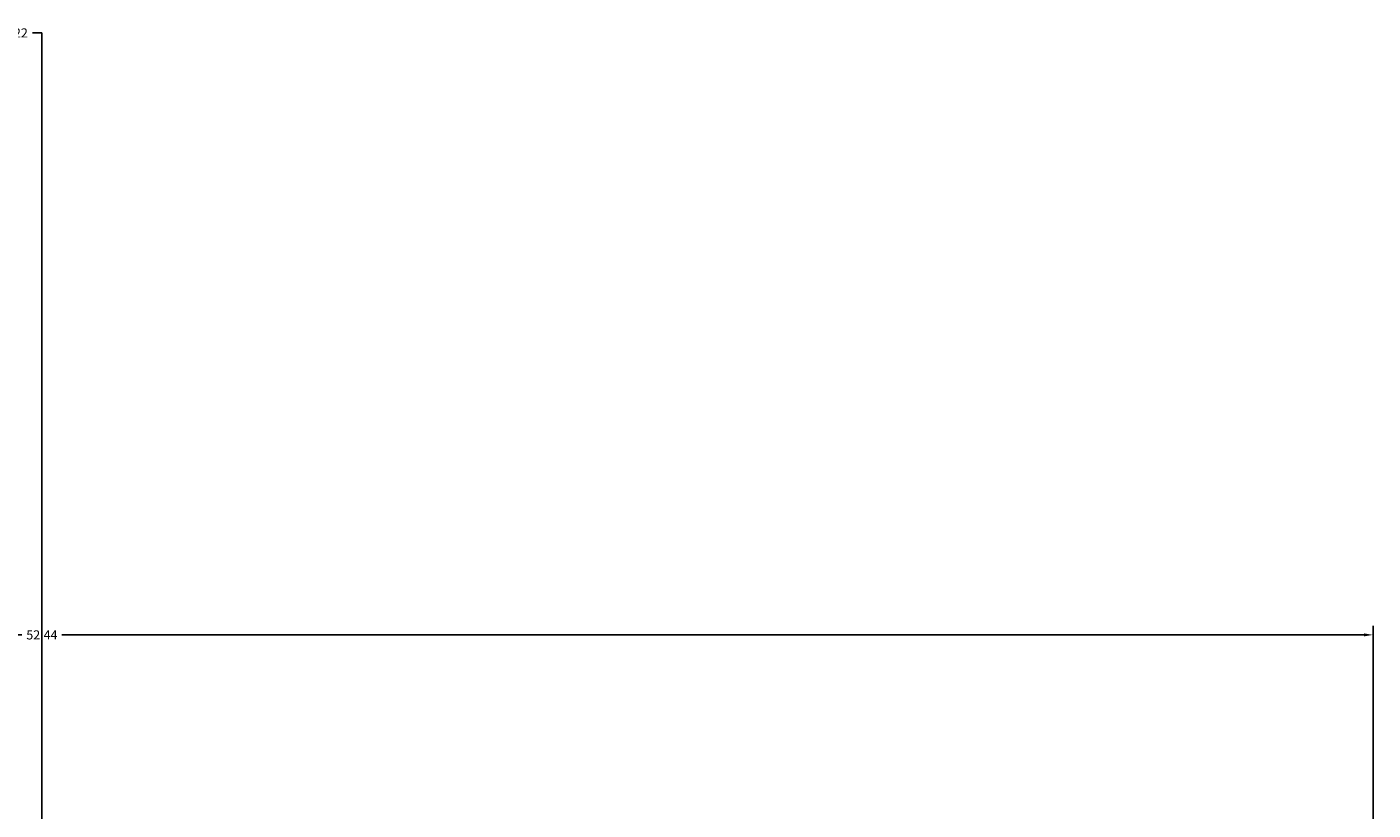
# Model space of a CAD drawing. Units: inches. Extents: x 12532.3 to 12594.9, y 6967.5 to 7063.
# Tile 9 of 9: x 12562.4 to 12588.9, y 7047.6 to 7063. Entities that reach past the tile are written whole.
import ezdxf

# ---------------------------------------------------------------- set-up
doc = ezdxf.new("R2010")
doc.units = ezdxf.units.IN
doc.header["$MEASUREMENT"] = 0
doc.header["$PDMODE"] = 98
doc.layers.add('A-ANNO-DIMS', color=2, linetype='Continuous', lineweight=18)
doc.styles.get("Standard").update_dxf_attribs({"font": 'arial.ttf'})
doc.dimstyles.get("Standard").update_dxf_attribs({"dimtxt": 0.18, "dimasz": 0.18, "dimexe": 0.18, "dimexo": 0.0625, "dimgap": 0.09, "dimtad": 0, "dimtih": 1, "dimtoh": 1, "dimdec": 4, "dimzin": 0, "dimdsep": 46, "dimtxsty": 'Standard', "dimcen": 0.09, "dimadec": 0, "dimazin": 0, "dimtfac": 1, "dimtdec": 4, "dimtofl": 0, "dimtmove": 0, "dimatfit": 3, "dimfxl": 1, "dimtolj": 1, "dimtzin": 0, "dimarcsym": 0})

# ---------------------------------------------------------------- blocks, each defined once
blk = doc.blocks.new('*D31')
at = {"layer": 'A-ANNO-DIMS', "color": 0, "lineweight": -2, "transparency": 16777216}
for p, q in [((12536.45, 7020.991), (12536.45, 7051.211)), ((12588.894, 7020.991), (12588.894, 7051.211)), ((12536.63, 7051.031), (12562.279, 7051.031)), ((12588.714, 7051.031), (12563.065, 7051.031))]:
    blk.add_line(p, q, dxfattribs=at)
at = {"layer": 'A-ANNO-DIMS', "color": 0, "transparency": 16777216}
for points in [[(12536.63, 7051.061), (12536.63, 7051.001), (12536.45, 7051.031)], [(12588.714, 7051.061), (12588.714, 7051.001), (12588.894, 7051.031)]]:
    blk.add_solid(points, dxfattribs=at)
at = {"layer": 'Defpoints', "color": 0, "transparency": 16777216}
for p in [(12588.894, 7051.031), (12536.45, 7020.929), (12588.894, 7020.929)]:
    blk.add_point(p, dxfattribs=at)
at = {"layer": 'A-ANNO-DIMS', "color": 0, "transparency": 16777216, "insert": (12562.672, 7051.031), "char_height": 0.18, "attachment_point": 5}
blk.add_mtext('\\A1;52.44', dxfattribs=at)
blk = doc.blocks.new('*D62')
at = {"layer": 'A-ANNO-DIMS', "color": 0, "lineweight": -2, "transparency": 16777216}
for p, q in [((12562.489, 7062.884), (12562.669, 7062.884)), ((12562.669, 7062.884), (12562.67, 7047.331)), ((12562.582, 7020.929), (12562.762, 7020.929)), ((12562.672, 7020.839), (12562.672, 7021.019))]:
    blk.add_line(p, q, dxfattribs=at)
at = {"layer": 'A-ANNO-DIMS', "color": 0, "transparency": 16777216}
blk.add_solid([(12562.7, 7047.331), (12562.64, 7047.331), (12562.67, 7047.151)], dxfattribs=at)
at = {"layer": 'Defpoints', "color": 0, "transparency": 16777216}
for p in [(12562.67, 7047.151), (12562.672, 7020.929)]:
    blk.add_point(p, dxfattribs=at)
at = {"layer": 'A-ANNO-DIMS', "color": 0, "transparency": 16777216, "insert": (12562.01, 7062.884), "char_height": 0.18, "attachment_point": 5}
blk.add_mtext('\\A1;R26.22', dxfattribs=at)

msp = doc.modelspace()

# ---------------------------------------------------------------- dimensions: what is measured, and where the dimension line sits
at = {"layer": 'A-ANNO-DIMS'}
dim = msp.add_radius_dim(center=(12562.6721, 7020.9287), mpoint=(12562.67, 7047.1506), dimstyle='Standard', override={"dimdec": 2, "dimlfac": 1, "dimrnd": 0, "dimzin": 0, "dimdsep": 46, "dimlunit": 2}, dxfattribs=at)
dim.commit()
dim.dimension.update_dxf_attribs({"geometry": '*D62', "text_midpoint": (12562.0098, 7062.8838), "dimtype": 164})
dim = msp.add_linear_dim(base=(12588.894, 7051.0306), p1=(12536.4501, 7020.9287), p2=(12588.894, 7020.9287), dimstyle='Standard', override={"dimdec": 2, "dimlfac": 1, "dimrnd": 0, "dimzin": 0, "dimdsep": 46, "dimlunit": 2}, dxfattribs=at)
dim.commit()
dim.dimension.update_dxf_attribs({"geometry": '*D31', "text_midpoint": (12562.6721, 7051.0306)})

doc.saveas('drawing.dxf')
